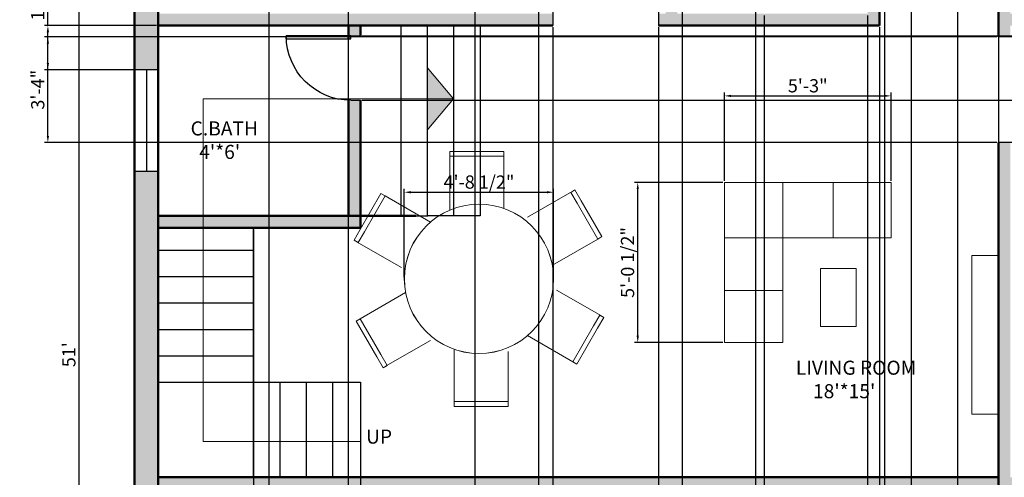
# Model space of a CAD drawing. Units: inches. Extents: x 2152 to 2718, y 1095 to 1798.
# Tile 3 of 5: x 2152 to 2524, y 1394 to 1567. Entities that reach past the tile are written whole.
import ezdxf

# ---------------------------------------------------------------- set-up
doc = ezdxf.new("R2010")
doc.units = ezdxf.units.IN
for name, color, linetype, lineweight in [('A-ANNO-DIMS', 130, 'Continuous', 18), ('A-ANNO-SYMB', 7, 'Continuous', 18), ('A-ANNO-TEXT', 130, 'Continuous', 18), ('A-AREA-IDEN', 130, 'Continuous', 25), ('A-FLOR-STRS', 7, 'Continuous', 25), ('A-WALL-PATT', 210, 'Continuous', 13), ('DOOR', 160, 'Continuous', 25), ('FUR', 10, 'Continuous', 18), ('WALL', 7, 'Continuous', 50), ('WIND', 140, 'Continuous', 25)]:
    doc.layers.add(name, color=color, linetype=linetype, lineweight=lineweight)
doc.styles.get("Standard").update_dxf_attribs({"font": 'arial.ttf'})
doc.dimstyles.new('ISO-25', dxfattribs={"dimtxt": 5, "dimasz": 2.5, "dimexe": 1.25, "dimexo": 0.625, "dimtad": 1, "dimdec": 0, "dimlunit": 4, "dimtxsty": 'Standard', "dimcen": 2.5, "dimadec": 0, "dimazin": 0, "dimtfac": 1, "dimtdec": 0, "dimtmove": 0, "dimatfit": 3, "dimfxl": 1, "dimarcsym": 0})

# ---------------------------------------------------------------- blocks, each defined once
blk = doc.blocks.new('*U2')
for p, q in [((0, 0), (0, -6)), ((40, 0), (40, -6))]:
    blk.add_line(p, q)
blk.add_lwpolyline([(0, 0), (0, 40), (1.75, 40), (1.75, 0)], close=True)
blk.add_arc((0, 0), 40, 0, 90)
blk = doc.blocks.new('*U9')
for p, q in [((-6.25, 38.26), (-10.99, 38.26)), ((-10.99, 38.26), (-10.99, 36.46)), ((-6.25, 38.26), (9.41, 38.26)), ((9.41, 38.26), (9.41, 36.46)), ((-10.99, 17.55), (-10.99, 37.14)), ((-6.25, 36.46), (-10.99, 36.46)), ((9.41, 36.46), (-6.25, 36.46)), ((9.41, 16.64), (9.41, 36.46))]:
    blk.add_line(p, q)
blk.add_circle((0, -10.01), 28.26)
blk = doc.blocks.new('*U10')
at = {"layer": 'FUR', "transparency": 16777216}
for p, rotation in [((2407.35, 1488.61), 59.99999999999999), ((2424.68, 1488.61), 300), ((2407.35, 1478.6), 120), ((2424.68, 1478.6), 240), ((2416.01, 1473.6), 180)]:
    blk.add_blockref('*U9', p, dxfattribs=dict(at, rotation=rotation))
blk.add_blockref('*U9', (2416.01, 1493.61), dxfattribs=at)
blk = doc.blocks.new('*D14')
at = {"layer": 'A-ANNO-DIMS', "color": 0, "lineweight": -2, "transparency": 16777216}
for p, q in [((2194.43, 1746.37), (2172.77, 1746.37)), ((2174.02, 1743.87), (2174.02, 1136.72)), ((2194.43, 1134.22), (2172.77, 1134.22))]:
    blk.add_line(p, q, dxfattribs=at)
at = {"layer": 'A-ANNO-DIMS', "color": 0, "transparency": 16777216}
for points in [[(2173.6, 1743.87), (2174.43, 1743.87), (2174.02, 1746.37)], [(2173.6, 1136.72), (2174.43, 1136.72), (2174.02, 1134.22)]]:
    blk.add_solid(points, dxfattribs=at)
at = {"layer": 'Defpoints', "color": 0, "transparency": 16777216}
for p in [(2195.06, 1746.37), (2174.02, 1134.22), (2195.06, 1134.22)]:
    blk.add_point(p, dxfattribs=at)
at = {"layer": 'A-ANNO-DIMS', "color": 0, "transparency": 16777216, "insert": (2170.84, 1440.29), "char_height": 5, "attachment_point": 5, "rotation": 90}
blk.add_mtext("51'", dxfattribs=at)
blk = doc.blocks.new('WIN-NARROW')
blk.add_line((0, 4.5), (38.45, 4.5))
blk.add_lwpolyline([(0, 0), (38.45, 0), (38.45, 9), (0, 9)], close=True)
blk = doc.blocks.new('*D36')
at = {"layer": 'A-ANNO-DIMS', "color": 0, "lineweight": -2, "transparency": 16777216}
for p, q in [((2204.06, 1736.74), (2204.06, 1098.09)), ((2275.93, 1736.74), (2275.93, 1098.09)), ((2206.56, 1099.34), (2273.43, 1099.34))]:
    blk.add_line(p, q, dxfattribs=at)
at = {"layer": 'A-ANNO-DIMS', "color": 0, "transparency": 16777216}
for points in [[(2206.56, 1099.75), (2206.56, 1098.92), (2204.06, 1099.34)], [(2273.43, 1099.75), (2273.43, 1098.92), (2275.93, 1099.34)]]:
    blk.add_solid(points, dxfattribs=at)
at = {"layer": 'Defpoints', "color": 0, "transparency": 16777216}
for p in [(2204.06, 1737.37), (2275.93, 1737.37), (2275.93, 1099.34)]:
    blk.add_point(p, dxfattribs=at)
at = {"layer": 'A-ANNO-DIMS', "color": 0, "transparency": 16777216, "insert": (2240, 1102.51), "char_height": 5, "attachment_point": 5}
blk.add_mtext('6\'-0"', dxfattribs=at)
blk = doc.blocks.new('*D40')
at = {"layer": 'A-ANNO-DIMS', "color": 0, "lineweight": -2, "transparency": 16777216}
for p, q in [((2162.26, 1564.87), (2162.26, 1593.09)), ((2203.43, 1564.87), (2161.01, 1564.87)), ((2162.26, 1550.66), (2162.26, 1562.37)), ((2203.43, 1548.16), (2161.01, 1548.16))]:
    blk.add_line(p, q, dxfattribs=at)
at = {"layer": 'A-ANNO-DIMS', "color": 0, "transparency": 16777216}
for points in [[(2161.84, 1562.37), (2162.68, 1562.37), (2162.26, 1564.87)], [(2161.84, 1550.66), (2162.68, 1550.66), (2162.26, 1548.16)]]:
    blk.add_solid(points, dxfattribs=at)
at = {"layer": 'Defpoints', "color": 0, "transparency": 16777216}
for p in [(2162.26, 1564.87), (2204.06, 1564.87), (2204.06, 1548.16)]:
    blk.add_point(p, dxfattribs=at)
at = {"layer": 'A-ANNO-DIMS', "color": 0, "transparency": 16777216, "insert": (2159.05, 1580.23), "char_height": 5, "attachment_point": 5, "rotation": 90}
blk.add_mtext('1\'-4 1/2"', dxfattribs=at)
blk = doc.blocks.new('*D42')
at = {"layer": 'A-ANNO-DIMS', "color": 0, "lineweight": -2, "transparency": 16777216}
for p, q in [((2204.06, 1176.99), (2204.06, 1788.86)), ((2206.56, 1787.61), (2243.52, 1787.61)), ((2246.02, 1176.99), (2246.02, 1788.86))]:
    blk.add_line(p, q, dxfattribs=at)
at = {"layer": 'A-ANNO-DIMS', "color": 0, "transparency": 16777216}
for points in [[(2206.56, 1788.03), (2206.56, 1787.19), (2204.06, 1787.61)], [(2243.52, 1788.03), (2243.52, 1787.19), (2246.02, 1787.61)]]:
    blk.add_solid(points, dxfattribs=at)
at = {"layer": 'Defpoints', "color": 0, "transparency": 16777216}
for p in [(2246.02, 1787.61), (2204.06, 1176.37), (2246.02, 1176.37)]:
    blk.add_point(p, dxfattribs=at)
at = {"layer": 'A-ANNO-DIMS', "color": 0, "transparency": 16777216, "insert": (2225.04, 1790.79), "char_height": 5, "attachment_point": 5}
blk.add_mtext('3\'-6"', dxfattribs=at)
blk = doc.blocks.new('*D45')
at = {"layer": 'A-ANNO-DIMS', "color": 0, "lineweight": -2, "transparency": 16777216}
for p, q in [((2204.06, 1487.74), (2204.06, 1098.09)), ((2240.06, 1487.74), (2240.06, 1098.09)), ((2206.56, 1099.34), (2237.56, 1099.34))]:
    blk.add_line(p, q, dxfattribs=at)
at = {"layer": 'A-ANNO-DIMS', "color": 0, "transparency": 16777216}
for points in [[(2206.56, 1099.75), (2206.56, 1098.92), (2204.06, 1099.34)], [(2237.56, 1099.75), (2237.56, 1098.92), (2240.06, 1099.34)]]:
    blk.add_solid(points, dxfattribs=at)
at = {"layer": 'Defpoints', "color": 0, "transparency": 16777216}
for p in [(2204.06, 1488.37), (2240.06, 1488.37), (2240.06, 1099.34)]:
    blk.add_point(p, dxfattribs=at)
at = {"layer": 'A-ANNO-DIMS', "color": 0, "transparency": 16777216, "insert": (2222.06, 1102.51), "char_height": 5, "attachment_point": 5}
blk.add_mtext('3\'-0"', dxfattribs=at)
blk = doc.blocks.new('*D50')
at = {"layer": 'A-ANNO-DIMS', "color": 0, "lineweight": -2, "transparency": 16777216}
for p, q in [((2707.86, 1560.98), (2707.86, 1589.76)), ((2281.18, 1560.98), (2709.11, 1560.98)), ((2707.86, 1539.09), (2707.86, 1558.48)), ((2281.18, 1536.59), (2709.11, 1536.59))]:
    blk.add_line(p, q, dxfattribs=at)
at = {"layer": 'A-ANNO-DIMS', "color": 0, "transparency": 16777216}
for points in [[(2707.44, 1558.48), (2708.28, 1558.48), (2707.86, 1560.98)], [(2707.44, 1539.09), (2708.28, 1539.09), (2707.86, 1536.59)]]:
    blk.add_solid(points, dxfattribs=at)
at = {"layer": 'Defpoints', "color": 0, "transparency": 16777216}
for p in [(2280.56, 1560.98), (2707.86, 1560.98), (2280.56, 1536.59)]:
    blk.add_point(p, dxfattribs=at)
at = {"layer": 'A-ANNO-DIMS', "color": 0, "transparency": 16777216, "insert": (2704.65, 1576.62), "char_height": 5, "attachment_point": 5, "rotation": 90}
blk.add_mtext('2\'-0 1/2"', dxfattribs=at)
blk = doc.blocks.new('*D52')
at = {"layer": 'A-ANNO-DIMS', "color": 0, "lineweight": -2, "transparency": 16777216}
for p, q in [((2402.42, 1648.24), (2402.42, 1098.09)), ((2430.09, 1648.24), (2430.09, 1098.09)), ((2404.92, 1099.34), (2427.59, 1099.34))]:
    blk.add_line(p, q, dxfattribs=at)
at = {"layer": 'A-ANNO-DIMS', "color": 0, "transparency": 16777216}
for points in [[(2404.92, 1099.75), (2404.92, 1098.92), (2402.42, 1099.34)], [(2427.59, 1099.75), (2427.59, 1098.92), (2430.09, 1099.34)]]:
    blk.add_solid(points, dxfattribs=at)
at = {"layer": 'Defpoints', "color": 0, "transparency": 16777216}
for p in [(2402.42, 1648.87), (2430.09, 1648.87), (2430.09, 1099.34)]:
    blk.add_point(p, dxfattribs=at)
at = {"layer": 'A-ANNO-DIMS', "color": 0, "transparency": 16777216, "insert": (2416.26, 1102.55), "char_height": 5, "attachment_point": 5}
blk.add_mtext('2\'-3 1/2"', dxfattribs=at)
blk = doc.blocks.new('*D53')
at = {"layer": 'A-ANNO-DIMS', "color": 0, "lineweight": -2, "transparency": 16777216}
for p, q in [((2353.45, 1564.24), (2353.45, 1098.09)), ((2393.45, 1564.24), (2393.45, 1098.09)), ((2355.95, 1099.34), (2390.95, 1099.34))]:
    blk.add_line(p, q, dxfattribs=at)
at = {"layer": 'A-ANNO-DIMS', "color": 0, "transparency": 16777216}
for points in [[(2355.95, 1099.75), (2355.95, 1098.92), (2353.45, 1099.34)], [(2390.95, 1099.75), (2390.95, 1098.92), (2393.45, 1099.34)]]:
    blk.add_solid(points, dxfattribs=at)
at = {"layer": 'Defpoints', "color": 0, "transparency": 16777216}
for p in [(2353.45, 1564.87), (2393.45, 1564.87), (2393.45, 1099.34)]:
    blk.add_point(p, dxfattribs=at)
at = {"layer": 'A-ANNO-DIMS', "color": 0, "transparency": 16777216, "insert": (2373.45, 1102.51), "char_height": 5, "attachment_point": 5}
blk.add_mtext('3\'-4"', dxfattribs=at)
blk = doc.blocks.new('*D56')
at = {"layer": 'A-ANNO-DIMS', "color": 0, "lineweight": -2, "transparency": 16777216}
for p, q in [((2477.06, 1564.24), (2477.06, 1098.09)), ((2522.06, 1564.24), (2522.06, 1098.09)), ((2479.56, 1099.34), (2519.56, 1099.34))]:
    blk.add_line(p, q, dxfattribs=at)
at = {"layer": 'A-ANNO-DIMS', "color": 0, "transparency": 16777216}
for points in [[(2479.56, 1099.75), (2479.56, 1098.92), (2477.06, 1099.34)], [(2519.56, 1099.75), (2519.56, 1098.92), (2522.06, 1099.34)]]:
    blk.add_solid(points, dxfattribs=at)
at = {"layer": 'Defpoints', "color": 0, "transparency": 16777216}
for p in [(2477.06, 1564.87), (2522.06, 1564.87), (2522.06, 1099.34)]:
    blk.add_point(p, dxfattribs=at)
at = {"layer": 'A-ANNO-DIMS', "color": 0, "transparency": 16777216, "insert": (2499.56, 1102.51), "char_height": 5, "attachment_point": 5}
blk.add_mtext('3\'-9"', dxfattribs=at)
blk = doc.blocks.new('*D57')
at = {"layer": 'A-ANNO-DIMS', "color": 0, "lineweight": -2, "transparency": 16777216}
for p, q in [((2489.06, 1721.19), (2489.06, 1098.09)), ((2522.06, 1710.69), (2522.06, 1098.09)), ((2491.56, 1099.34), (2519.56, 1099.34))]:
    blk.add_line(p, q, dxfattribs=at)
at = {"layer": 'A-ANNO-DIMS', "color": 0, "transparency": 16777216}
for points in [[(2491.56, 1099.75), (2491.56, 1098.92), (2489.06, 1099.34)], [(2519.56, 1099.75), (2519.56, 1098.92), (2522.06, 1099.34)]]:
    blk.add_solid(points, dxfattribs=at)
at = {"layer": 'Defpoints', "color": 0, "transparency": 16777216}
for p in [(2489.06, 1721.81), (2522.06, 1711.31), (2522.06, 1099.34)]:
    blk.add_point(p, dxfattribs=at)
at = {"layer": 'A-ANNO-DIMS', "color": 0, "transparency": 16777216, "insert": (2505.56, 1102.51), "char_height": 5, "attachment_point": 5}
blk.add_mtext('2\'-9"', dxfattribs=at)
blk = doc.blocks.new('*D59')
at = {"layer": 'A-ANNO-DIMS', "color": 0, "lineweight": -2, "transparency": 16777216}
for p, q in [((2478.92, 1660.24), (2478.92, 1098.09)), ((2506.58, 1660.24), (2506.58, 1098.09)), ((2481.42, 1099.34), (2504.08, 1099.34))]:
    blk.add_line(p, q, dxfattribs=at)
at = {"layer": 'A-ANNO-DIMS', "color": 0, "transparency": 16777216}
for points in [[(2481.42, 1099.75), (2481.42, 1098.92), (2478.92, 1099.34)], [(2504.08, 1099.75), (2504.08, 1098.92), (2506.58, 1099.34)]]:
    blk.add_solid(points, dxfattribs=at)
at = {"layer": 'Defpoints', "color": 0, "transparency": 16777216}
for p in [(2478.92, 1660.87), (2506.58, 1660.87), (2506.58, 1099.34)]:
    blk.add_point(p, dxfattribs=at)
at = {"layer": 'A-ANNO-DIMS', "color": 0, "transparency": 16777216, "insert": (2492.75, 1102.55), "char_height": 5, "attachment_point": 5}
blk.add_mtext('2\'-3 1/2"', dxfattribs=at)
blk = doc.blocks.new('*D60')
at = {"layer": 'A-ANNO-DIMS', "color": 0, "lineweight": -2, "transparency": 16777216}
for p, q in [((2433.42, 1568.74), (2433.42, 1098.09)), ((2472.56, 1568.74), (2472.56, 1098.09)), ((2435.92, 1099.34), (2470.06, 1099.34))]:
    blk.add_line(p, q, dxfattribs=at)
at = {"layer": 'A-ANNO-DIMS', "color": 0, "transparency": 16777216}
for points in [[(2435.92, 1099.75), (2435.92, 1098.92), (2433.42, 1099.34)], [(2470.06, 1099.75), (2470.06, 1098.92), (2472.56, 1099.34)]]:
    blk.add_solid(points, dxfattribs=at)
at = {"layer": 'Defpoints', "color": 0, "transparency": 16777216}
for p in [(2433.42, 1569.37), (2472.56, 1569.37), (2472.56, 1099.34)]:
    blk.add_point(p, dxfattribs=at)
at = {"layer": 'A-ANNO-DIMS', "color": 0, "transparency": 16777216, "insert": (2452.99, 1102.51), "char_height": 5, "attachment_point": 5}
blk.add_mtext('3\'-3"', dxfattribs=at)
blk = doc.blocks.new('*D65')
at = {"layer": 'A-ANNO-DIMS', "color": 0, "lineweight": -2, "transparency": 16777216}
for p, q in [((2418.35, 1506.09), (2418.35, 1539.52)), ((2481.44, 1506.09), (2481.44, 1539.52)), ((2420.85, 1538.27), (2478.94, 1538.27))]:
    blk.add_line(p, q, dxfattribs=at)
at = {"layer": 'A-ANNO-DIMS', "color": 0, "transparency": 16777216}
for points in [[(2420.85, 1538.69), (2420.85, 1537.85), (2418.35, 1538.27)], [(2478.94, 1538.69), (2478.94, 1537.85), (2481.44, 1538.27)]]:
    blk.add_solid(points, dxfattribs=at)
at = {"layer": 'Defpoints', "color": 0, "transparency": 16777216}
for p in [(2481.44, 1538.27), (2418.35, 1505.47), (2481.44, 1505.47)]:
    blk.add_point(p, dxfattribs=at)
at = {"layer": 'A-ANNO-DIMS', "color": 0, "transparency": 16777216, "insert": (2449.9, 1541.45), "char_height": 5, "attachment_point": 5}
blk.add_mtext('5\'-3"', dxfattribs=at)
blk = doc.blocks.new('*D66')
at = {"layer": 'A-ANNO-DIMS', "color": 0, "lineweight": -2, "transparency": 16777216}
for p, q in [((2417.72, 1505.47), (2384.3, 1505.47)), ((2385.55, 1447.43), (2385.55, 1502.97)), ((2417.72, 1444.93), (2384.3, 1444.93))]:
    blk.add_line(p, q, dxfattribs=at)
at = {"layer": 'A-ANNO-DIMS', "color": 0, "transparency": 16777216}
for points in [[(2385.13, 1502.97), (2385.97, 1502.97), (2385.55, 1505.47)], [(2385.13, 1447.43), (2385.97, 1447.43), (2385.55, 1444.93)]]:
    blk.add_solid(points, dxfattribs=at)
at = {"layer": 'Defpoints', "color": 0, "transparency": 16777216}
for p in [(2385.55, 1505.47), (2418.35, 1505.47), (2418.35, 1444.93)]:
    blk.add_point(p, dxfattribs=at)
at = {"layer": 'A-ANNO-DIMS', "color": 0, "transparency": 16777216, "insert": (2382.34, 1475.2), "char_height": 5, "attachment_point": 5, "rotation": 90}
blk.add_mtext('5\'-0 1/2"', dxfattribs=at)
blk = doc.blocks.new('*D67')
at = {"layer": 'A-ANNO-DIMS', "color": 0, "lineweight": -2, "transparency": 16777216}
for p, q in [((2297.19, 1469.62), (2297.19, 1503.04)), ((2353.71, 1469.62), (2353.71, 1503.04)), ((2299.69, 1501.79), (2351.21, 1501.79))]:
    blk.add_line(p, q, dxfattribs=at)
at = {"layer": 'A-ANNO-DIMS', "color": 0, "transparency": 16777216}
for points in [[(2299.69, 1502.21), (2299.69, 1501.37), (2297.19, 1501.79)], [(2351.21, 1502.21), (2351.21, 1501.37), (2353.71, 1501.79)]]:
    blk.add_solid(points, dxfattribs=at)
at = {"layer": 'Defpoints', "color": 0, "transparency": 16777216}
for p in [(2353.71, 1501.79), (2297.19, 1468.99), (2353.71, 1468.99)]:
    blk.add_point(p, dxfattribs=at)
at = {"layer": 'A-ANNO-DIMS', "color": 0, "transparency": 16777216, "insert": (2325.45, 1505), "char_height": 5, "attachment_point": 5}
blk.add_mtext('4\'-8 1/2"', dxfattribs=at)
blk = doc.blocks.new('*D68')
at = {"layer": 'A-ANNO-DIMS', "color": 0, "lineweight": -2, "transparency": 16777216}
for p, q in [((2324.06, 1258.93), (2324.06, 1788.86)), ((2326.56, 1787.61), (2345.56, 1787.61)), ((2348.06, 1258.93), (2348.06, 1788.86))]:
    blk.add_line(p, q, dxfattribs=at)
at = {"layer": 'A-ANNO-DIMS', "color": 0, "transparency": 16777216}
for points in [[(2326.56, 1788.03), (2326.56, 1787.19), (2324.06, 1787.61)], [(2345.56, 1788.03), (2345.56, 1787.19), (2348.06, 1787.61)]]:
    blk.add_solid(points, dxfattribs=at)
at = {"layer": 'Defpoints', "color": 0, "transparency": 16777216}
for p in [(2348.06, 1787.61), (2324.06, 1258.3), (2348.06, 1258.3)]:
    blk.add_point(p, dxfattribs=at)
at = {"layer": 'A-ANNO-DIMS', "color": 0, "transparency": 16777216, "insert": (2336.06, 1790.79), "char_height": 5, "attachment_point": 5}
blk.add_mtext('2\'-0"', dxfattribs=at)
blk = doc.blocks.new('*D69')
at = {"layer": 'A-ANNO-DIMS', "color": 0, "lineweight": -2, "transparency": 16777216}
for p, q in [((2521.43, 1560.6), (2161.01, 1560.6)), ((2162.26, 1523.1), (2162.26, 1558.1)), ((2521.43, 1520.6), (2161.01, 1520.6))]:
    blk.add_line(p, q, dxfattribs=at)
at = {"layer": 'A-ANNO-DIMS', "color": 0, "transparency": 16777216}
for points in [[(2161.84, 1558.1), (2162.68, 1558.1), (2162.26, 1560.6)], [(2161.84, 1523.1), (2162.68, 1523.1), (2162.26, 1520.6)]]:
    blk.add_solid(points, dxfattribs=at)
at = {"layer": 'Defpoints', "color": 0, "transparency": 16777216}
for p in [(2162.26, 1560.6), (2522.06, 1560.6), (2522.06, 1520.6)]:
    blk.add_point(p, dxfattribs=at)
at = {"layer": 'A-ANNO-DIMS', "color": 0, "transparency": 16777216, "insert": (2159.08, 1540.6), "char_height": 5, "attachment_point": 5, "rotation": 90}
blk.add_mtext('3\'-4"', dxfattribs=at)

msp = doc.modelspace()

# ---------------------------------------------------------------- hatches: boundary and pattern name
at = {"layer": 'A-ANNO-SYMB'}
h = msp.add_hatch(color=256, dxfattribs=at)
h.dxf.hatch_style = 1
h.paths.add_polyline_path([(2305.86, 1549), (2305.86, 1537.12), (2315.86, 1537.12)])
h.paths.add_polyline_path([(2315.86, 1537.12), (2305.86, 1537.12), (2305.86, 1525.24)])
at = {"layer": 'A-WALL-PATT'}
h = msp.add_hatch(color=256, dxfattribs=at)
h.dxf.hatch_style = 1
h.paths.add_polyline_path([(2204.06, 1737.37), (2275.93, 1737.37), (2275.93, 1746.37), (2195.06, 1746.37), (2195.06, 1548.16), (2204.06, 1548.16)])
h.paths.add_polyline_path([(2567.46, 1746.37), (2519.79, 1746.37), (2519.79, 1737.37), (2549.06, 1737.37), (2567.46, 1737.37)])
h.paths.add_polyline_path([(2526.56, 1706.63), (2526.56, 1737.37), (2522.06, 1737.37), (2522.06, 1614.04), (2526.56, 1614.04), (2526.56, 1660.87)])
h.paths.add_polyline_path([(2477.06, 1737.37), (2472.56, 1737.37), (2472.56, 1653.37), (2430.09, 1653.37), (2430.09, 1648.87), (2472.56, 1648.87), (2472.56, 1569.37), (2400.56, 1569.37), (2400.56, 1573.72), (2399.94, 1573.72), (2396.06, 1573.72), (2396.06, 1569.37), (2393.45, 1569.37), (2393.45, 1564.87), (2477.06, 1564.87), (2477.06, 1648.87)])
h.paths.add_polyline_path([(2400.56, 1737.37), (2396.06, 1737.37), (2396.06, 1599.61), (2400.56, 1599.61), (2400.56, 1648.87), (2402.42, 1648.87), (2402.42, 1653.37), (2400.56, 1653.37)], flags=17)
h.paths.add_polyline_path([(2353.45, 1569.37), (2204.06, 1569.37), (2204.06, 1564.87), (2353.45, 1564.87)])
h.paths.add_polyline_path([(2280.56, 1492.87), (2221.07, 1492.87), (2221.07, 1488.37), (2280.56, 1488.37)])
h.paths.add_polyline_path([(2221.07, 1492.87), (2204.06, 1492.87), (2204.06, 1488.37), (2221.07, 1488.37)])
h.paths.add_polyline_path([(2280.56, 1536.59), (2276.9, 1536.59, -0.008622), (2276.06, 1536.6), (2276.06, 1492.87), (2280.56, 1492.87)])
h.paths.add_polyline_path([(2280.56, 1564.87), (2276.06, 1564.87), (2276.06, 1560.98), (2276.9, 1560.98), (2280.56, 1560.98)])
h.paths.add_polyline_path([(2675.06, 1746.37), (2630.54, 1746.37), (2630.54, 1737.37), (2666.06, 1737.37), (2666.06, 1384.87), (2675.06, 1384.87)])
h.paths.add_polyline_path([(2666.06, 1569.37), (2578.28, 1569.37), (2526.56, 1569.37), (2526.56, 1574.04), (2522.06, 1574.04), (2522.06, 1564.87), (2522.06, 1560.6), (2526.56, 1560.6), (2526.56, 1564.87), (2666.06, 1564.87)])
h.paths.add_polyline_path([(2526.56, 1520.6), (2522.06, 1520.6), (2522.06, 1384.87), (2570.2, 1384.87), (2570.2, 1393.87), (2526.56, 1393.87)])
h.paths.add_polyline_path([(2666.06, 1393.87), (2633.28, 1393.87), (2633.28, 1384.87), (2666.06, 1384.87)], flags=17)
h.paths.add_polyline_path([(2522.06, 1393.87), (2306.06, 1393.87), (2280.56, 1393.87), (2280.56, 1384.87), (2301.56, 1384.87), (2522.06, 1384.87)])
h.paths.add_polyline_path([(2280.56, 1393.87), (2204.06, 1393.87), (2204.06, 1384.87), (2232.43, 1384.87), (2280.56, 1384.87)])
h.paths.add_polyline_path([(2204.06, 1509.71), (2195.06, 1509.71), (2195.06, 1364.72), (2204.06, 1364.72), (2204.06, 1384.87)])
h.paths.add_polyline_path([(2204.06, 1326.27), (2195.06, 1326.27), (2195.06, 1302.62), (2201.06, 1302.62), (2204.06, 1302.62), (2204.06, 1308.37)])
h.paths.add_polyline_path([(2280.56, 1384.87), (2276.06, 1384.87), (2276.06, 1312.87), (2273.63, 1312.87), (2273.63, 1312.11), (2273.63, 1308.37), (2280.56, 1308.37)])
h.paths.add_polyline_path([(2248.67, 1312.11, -0.007577), (2248.69, 1312.87), (2204.06, 1312.87), (2204.06, 1308.37), (2248.67, 1308.37)])
h.paths.add_polyline_path([(2364.43, 1297.87), (2364.43, 1300.87), (2357.06, 1300.87), (2357.06, 1291.87), (2364.43, 1291.87)])
h.paths.add_polyline_path([(2428.34, 1300.87), (2404.32, 1300.87, -0.01877), (2404.43, 1297.87), (2404.43, 1291.87), (2428.34, 1291.87)])
h.paths.add_polyline_path([(2522.06, 1384.87), (2513.06, 1384.87), (2513.06, 1300.87), (2491.42, 1300.87), (2491.42, 1291.87), (2522.06, 1291.87)])
h.paths.add_polyline_path([(2357.06, 1384.87), (2348.06, 1384.87), (2348.06, 1176.37), (2309.1, 1176.37), (2309.1, 1167.37), (2357.06, 1167.37), (2357.06, 1173.65)])
h.paths.add_polyline_path([(2475.5, 1693.24), (2504.24, 1693.24), (2504.24, 1713.14), (2475.5, 1713.14)], flags=9)

# ---------------------------------------------------------------- linework, layer by layer
at = {"layer": 'A-ANNO-SYMB'}
for p, q in [((2315.86, 1537.12), (2305.86, 1549)), ((2221.07, 1407.37), (2221.07, 1537.12)), ((2221.07, 1537.12), (2315.86, 1537.12)), ((2315.86, 1537.12), (2305.86, 1525.24)), ((2280.56, 1407.37), (2221.07, 1407.37))]:
    msp.add_line(p, q, dxfattribs=at)
at = {"layer": 'A-FLOR-STRS'}
for p, q in [((2295.86, 1564.87), (2295.86, 1492.87)), ((2305.86, 1564.87), (2305.86, 1492.87)), ((2315.86, 1564.87), (2315.86, 1492.87)), ((2325.86, 1564.87), (2325.86, 1492.87)), ((2301.56, 1492.87), (2306.06, 1492.87)), ((2325.86, 1492.87), (2306.06, 1492.87)), ((2240.06, 1393.87), (2240.06, 1488.37)), ((2204.06, 1479.87), (2240.06, 1479.87)), ((2204.06, 1469.87), (2240.06, 1469.87)), ((2204.06, 1459.87), (2240.06, 1459.87)), ((2204.06, 1449.87), (2240.06, 1449.87)), ((2204.06, 1439.87), (2240.06, 1439.87)), ((2204.06, 1393.87), (2204.06, 1429.87)), ((2204.06, 1429.87), (2280.56, 1429.87)), ((2204.06, 1429.87), (2240.06, 1429.87)), ((2240.06, 1429.87), (2240.06, 1393.87)), ((2250.06, 1429.87), (2250.06, 1393.87)), ((2260.06, 1429.87), (2260.06, 1393.87)), ((2270.06, 1429.87), (2270.06, 1393.87)), ((2280.56, 1429.87), (2280.56, 1384.87)), ((2204.06, 1393.87), (2240.06, 1393.87))]:
    msp.add_line(p, q, dxfattribs=at)
at = {"layer": 'FUR'}
for p, q in [((2459.58, 1484.56), (2459.58, 1505.47)), ((2314.46, 1496.55), (2314.46, 1495.02)), ((2418.35, 1464.59), (2440.53, 1464.59))]:
    msp.add_line(p, q, dxfattribs=at)
for points in [[(2418.35, 1505.47), (2481.44, 1505.47), (2481.44, 1484.56), (2418.35, 1484.56)], [(2418.35, 1505.47), (2440.53, 1505.47), (2440.53, 1444.93), (2418.35, 1444.93)], [(2522.06, 1477.86), (2511.97, 1477.86), (2511.97, 1417.74), (2522.06, 1417.74)], [(2454.67, 1472.89), (2468.22, 1472.89), (2468.22, 1450.91), (2454.67, 1450.91)]]:
    msp.add_lwpolyline(points, close=True, dxfattribs=at)
at = {"layer": 'WALL'}
for p, q in [((2195.06, 1302.62), (2195.06, 1746.37)), ((2204.06, 1300.87), (2204.06, 1737.37)), ((2477.06, 1648.87), (2477.06, 1564.87)), ((2522.06, 1574.04), (2522.06, 1564.87)), ((2204.06, 1564.87), (2204.06, 1492.87)), ((2353.45, 1564.87), (2204.06, 1564.87)), ((2276.06, 1559.92), (2276.06, 1564.87)), ((2280.56, 1560.98), (2280.56, 1564.87)), ((2477.06, 1564.87), (2393.45, 1564.87)), ((2522.06, 1560.6), (2522.06, 1564.87)), ((2276.06, 1492.87), (2276.06, 1536.6)), ((2280.56, 1488.37), (2280.56, 1536.59)), ((2522.06, 1384.87), (2522.06, 1520.6)), ((2204.06, 1492.87), (2301.56, 1492.87)), ((2204.06, 1492.87), (2276.06, 1492.87)), ((2204.06, 1492.87), (2276.06, 1492.87)), ((2204.06, 1488.37), (2280.56, 1488.37)), ((2306.06, 1393.87), (2204.06, 1393.87)), ((2522.06, 1393.87), (2306.06, 1393.87))]:
    msp.add_line(p, q, dxfattribs=at)

# ---------------------------------------------------------------- block references
at = {"layer": 'DOOR', "xscale": -1}
msp.add_blockref('*U2', (2393.45, 1570.87), dxfattribs=at)
at = {"layer": 'DOOR', "xscale": -0.6098166643384796, "yscale": 0.6098166643384796, "zscale": 0.6098166643384796, "rotation": 90}
msp.add_blockref('*U2', (2276.9, 1560.98), dxfattribs=at)
at = {"layer": 'DOOR', "rotation": 270}
msp.add_blockref('*U2', (2528.06, 1560.6), dxfattribs=at)
at = {"layer": 'FUR'}
msp.add_blockref('*U10', (-90.56, -14.61), dxfattribs=at)
at = {"layer": 'WIND', "rotation": 270.0000000000007}
msp.add_blockref('WIN-NARROW', (2195.06, 1548.16), dxfattribs=at)

# ---------------------------------------------------------------- texts
at = {"layer": 'A-ANNO-TEXT', "insert": (2282.7, 1411.94), "char_height": 5.331, "attachment_point": 1}
msp.add_mtext_dynamic_manual_height_columns('UP', width=138.497, gutter_width=26.66, heights=[0], dxfattribs=at)
at = {"layer": 'A-AREA-IDEN', "attachment_point": 1}
for s, insert, char_height in [("C.BATH\\P  4'*6'", (2216.29, 1528.62), 5.331), ("LIVING ROOM\\P    18'*15'", (2445.38, 1438.02), 5.3311)]:
    msp.add_mtext_dynamic_manual_height_columns(s, width=138.497, gutter_width=26.66, heights=[0], dxfattribs=dict(at, insert=insert, char_height=char_height))

# ---------------------------------------------------------------- dimensions: what is measured, and where the dimension line sits
at = {"layer": 'A-ANNO-DIMS'}
for base, p1, p2, picture, middle in [((2246.02, 1787.61), (2204.06, 1176.37), (2246.02, 1176.37), '*D42', (2225.04, 1790.79)), ((2348.06, 1787.61), (2324.06, 1258.3), (2348.06, 1258.3), '*D68', (2336.06, 1790.79)), ((2275.93, 1099.34), (2204.06, 1737.37), (2275.93, 1737.37), '*D36', (2240, 1102.51)), ((2522.06, 1099.34), (2489.06, 1721.81), (2522.06, 1711.31), '*D57', (2505.56, 1102.51)), ((2506.58, 1099.34), (2478.92, 1660.87), (2506.58, 1660.87), '*D59', (2492.75, 1102.55)), ((2430.09, 1099.34), (2402.42, 1648.87), (2430.09, 1648.87), '*D52', (2416.26, 1102.55)), ((2472.56, 1099.34), (2433.42, 1569.37), (2472.56, 1569.37), '*D60', (2452.99, 1102.51)), ((2393.45, 1099.34), (2353.45, 1564.87), (2393.45, 1564.87), '*D53', (2373.45, 1102.51)), ((2522.06, 1099.34), (2477.06, 1564.87), (2522.06, 1564.87), '*D56', (2499.56, 1102.51)), ((2481.44, 1538.27), (2418.35, 1505.47), (2481.44, 1505.47), '*D65', (2449.9, 1541.45)), ((2353.71, 1501.79), (2297.19, 1468.99), (2353.71, 1468.99), '*D67', (2325.45, 1505)), ((2240.06, 1099.34), (2204.06, 1488.37), (2240.06, 1488.37), '*D45', (2222.06, 1102.51))]:
    dim = msp.add_linear_dim(base=base, p1=p1, p2=p2, dimstyle='ISO-25', override={"dimdec": 1, "dimlfac": 1, "dimrnd": 0, "dimzin": 1, "dimdsep": 46, "dimlunit": 4, "dimfrac": 2}, dxfattribs=at)
    dim.commit()
    dim.dimension.update_dxf_attribs({"geometry": picture, "text_midpoint": middle})
for base, p1, p2, override, picture, middle in [((2174.02, 1134.22), (2195.06, 1746.37), (2195.06, 1134.22), {"dimclrd": 0, "dimclre": 0, "dimclrt": 0}, '*D14', (2170.84, 1440.29)), ((2162.26, 1564.87), (2204.06, 1548.16), (2204.06, 1564.87), {"dimdec": 1, "dimlfac": 1, "dimrnd": 0, "dimzin": 1, "dimdsep": 46, "dimlunit": 4, "dimfrac": 2}, '*D40', (2159.05, 1580.23)), ((2707.86, 1560.98), (2280.56, 1536.59), (2280.56, 1560.98), {"dimdec": 1, "dimlfac": 1, "dimrnd": 0, "dimzin": 1, "dimdsep": 46, "dimlunit": 4, "dimfrac": 2}, '*D50', (2704.65, 1576.62)), ((2162.26, 1560.6), (2522.06, 1520.6), (2522.06, 1560.6), {"dimdec": 1, "dimlfac": 1, "dimrnd": 0, "dimzin": 1, "dimdsep": 46, "dimlunit": 4, "dimfrac": 2}, '*D69', (2159.08, 1540.6)), ((2385.55, 1505.47), (2418.35, 1444.93), (2418.35, 1505.47), {"dimdec": 1, "dimlfac": 1, "dimrnd": 0, "dimzin": 1, "dimdsep": 46, "dimlunit": 4, "dimfrac": 2}, '*D66', (2382.34, 1475.2))]:
    dim = msp.add_linear_dim(base=base, p1=p1, p2=p2, angle=90, dimstyle='ISO-25', override=override, dxfattribs=at)
    dim.commit()
    dim.dimension.update_dxf_attribs({"geometry": picture, "text_midpoint": middle})

doc.saveas('drawing.dxf')
